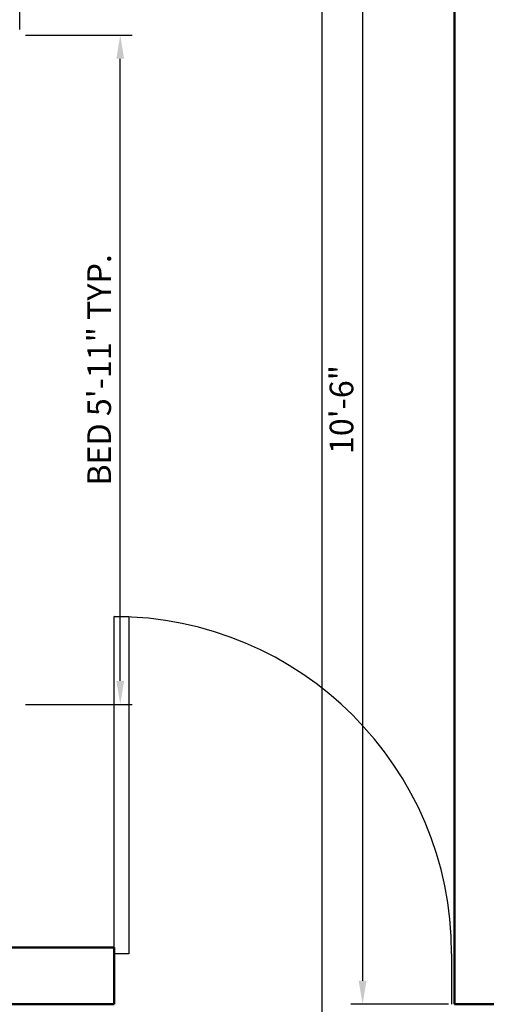
# Model space of a CAD drawing. Units: inches. Extents: x 2385 to 2740, y 1752 to 2305.
# Tile 9 of 15: x 2485 to 2535, y 2141 to 2245. Entities that reach past the tile are written whole.
import ezdxf

# ---------------------------------------------------------------- set-up
doc = ezdxf.new("R2010")
doc.units = ezdxf.units.IN
for name, color, linetype, lineweight in [('A-ANNO-DIMS', 2, 'Continuous', 18), ('A-DOOR', 4, 'Continuous', 25), ('A-WALL', 7, 'Continuous', 50)]:
    doc.layers.add(name, color=color, linetype=linetype, lineweight=lineweight)
doc.styles.get("Standard").update_dxf_attribs({"font": 'arial.ttf'})
doc.dimstyles.new('Copy of ISO-25', dxfattribs={"dimtxt": 2.5, "dimasz": 2.5, "dimexe": 1.25, "dimexo": 0.625, "dimtad": 1, "dimdec": 1, "dimlunit": 4, "dimtxsty": 'Standard', "dimcen": 2.5, "dimadec": 0, "dimazin": 0, "dimtfac": 1, "dimtdec": 1, "dimtmove": 0, "dimatfit": 3, "dimfxl": 1, "dimarcsym": 0})

# ---------------------------------------------------------------- blocks, each defined once
blk = doc.blocks.new('*D7')
at = {"layer": 'A-ANNO-DIMS', "color": 0, "lineweight": -2, "transparency": 16777216}
for p, q in [((2530.62, 2266.97), (2520.29, 2266.97)), ((2521.54, 2264.47), (2521.54, 2143.47)), ((2530.62, 2140.97), (2520.29, 2140.97))]:
    blk.add_line(p, q, dxfattribs=at)
at = {"layer": 'A-ANNO-DIMS', "color": 0, "transparency": 16777216}
for points in [[(2521.12, 2264.47), (2521.95, 2264.47), (2521.54, 2266.97)], [(2521.12, 2143.47), (2521.95, 2143.47), (2521.54, 2140.97)]]:
    blk.add_solid(points, dxfattribs=at)
at = {"layer": 'Defpoints', "color": 0, "transparency": 16777216}
for p in [(2531.25, 2266.97), (2521.54, 2140.97), (2531.25, 2140.97)]:
    blk.add_point(p, dxfattribs=at)
at = {"layer": 'A-ANNO-DIMS', "color": 0, "transparency": 16777216, "insert": (2519.63, 2203.97), "char_height": 2.5, "attachment_point": 5, "rotation": 90}
blk.add_mtext('10\'-6"', dxfattribs=at)
blk = doc.blocks.new('*U4')
for p, q in [((0, 0), (0, -6)), ((40, 0), (40, -6))]:
    blk.add_line(p, q)
blk.add_lwpolyline([(0, 0), (0, 40), (1.75, 40), (1.75, 0)], close=True)
blk.add_arc((0, 0), 40, 0, 90)
blk = doc.blocks.new('*D26')
at = {"layer": 'A-ANNO-DIMS', "color": 0, "lineweight": -2, "transparency": 16777216}
for p, q in [((2485.89, 2243.62), (2497.15, 2243.62)), ((2495.9, 2175.23), (2495.9, 2241.12)), ((2485.89, 2172.73), (2497.15, 2172.73))]:
    blk.add_line(p, q, dxfattribs=at)
at = {"layer": 'A-ANNO-DIMS', "color": 0, "transparency": 16777216}
for points in [[(2495.48, 2241.12), (2496.31, 2241.12), (2495.9, 2243.62)], [(2495.48, 2175.23), (2496.31, 2175.23), (2495.9, 2172.73)]]:
    blk.add_solid(points, dxfattribs=at)
at = {"layer": 'Defpoints', "color": 0, "transparency": 16777216}
for p in [(2485.26, 2243.62), (2495.9, 2243.62), (2485.26, 2172.73)]:
    blk.add_point(p, dxfattribs=at)
at = {"layer": 'A-ANNO-DIMS', "color": 0, "transparency": 16777216, "insert": (2493.99, 2208.17), "char_height": 2.5, "attachment_point": 5, "rotation": 90}
blk.add_mtext('BED 5\'-11" TYP.', dxfattribs=at)
blk = doc.blocks.new('*D27')
at = {"layer": 'A-ANNO-DIMS', "color": 0, "lineweight": -2, "transparency": 16777216}
for p, q in [((2429.86, 2244.24), (2429.86, 2255.5)), ((2485.26, 2244.24), (2485.26, 2255.5)), ((2482.76, 2254.25), (2432.36, 2254.25))]:
    blk.add_line(p, q, dxfattribs=at)
at = {"layer": 'A-ANNO-DIMS', "color": 0, "transparency": 16777216}
for points in [[(2432.36, 2254.67), (2432.36, 2253.84), (2429.86, 2254.25)], [(2482.76, 2254.67), (2482.76, 2253.84), (2485.26, 2254.25)]]:
    blk.add_solid(points, dxfattribs=at)
at = {"layer": 'Defpoints', "color": 0, "transparency": 16777216}
for p in [(2429.86, 2254.25), (2429.86, 2243.62), (2485.26, 2243.62)]:
    blk.add_point(p, dxfattribs=at)
at = {"layer": 'A-ANNO-DIMS', "color": 0, "transparency": 16777216, "insert": (2457.56, 2256.17), "char_height": 2.5, "attachment_point": 5}
blk.add_mtext('4\'-7 1/2" TYP.', dxfattribs=at)
blk = doc.blocks.new('*D48')
at = {"layer": 'A-ANNO-DIMS', "color": 0, "lineweight": -2, "transparency": 16777216}
for p, q in [((2517.25, 1916.59), (2517.25, 2302.84)), ((2553.25, 1916.59), (2553.25, 2302.84)), ((2519.75, 2301.59), (2550.75, 2301.59))]:
    blk.add_line(p, q, dxfattribs=at)
at = {"layer": 'A-ANNO-DIMS', "color": 0, "transparency": 16777216}
for points in [[(2519.75, 2302), (2519.75, 2301.17), (2517.25, 2301.59)], [(2550.75, 2302), (2550.75, 2301.17), (2553.25, 2301.59)]]:
    blk.add_solid(points, dxfattribs=at)
at = {"layer": 'Defpoints', "color": 0, "transparency": 16777216}
for p in [(2553.25, 2301.59), (2517.25, 1915.97), (2553.25, 1915.97)]:
    blk.add_point(p, dxfattribs=at)
at = {"layer": 'A-ANNO-DIMS', "color": 0, "transparency": 16777216, "insert": (2535.25, 2303.49), "char_height": 2.5, "attachment_point": 5}
blk.add_mtext('3\'-0"', dxfattribs=at)

msp = doc.modelspace()

# ---------------------------------------------------------------- linework, layer by layer
at = {"layer": 'A-WALL'}
for p, q in [((2531.25, 2146.97), (2531.25, 2266.97)), ((2423.25, 2146.97), (2495.25, 2146.97)), ((2495.25, 2140.97), (2495.25, 2146.97)), ((2531.25, 2146.97), (2531.25, 2140.97)), ((2495.25, 2140.97), (2423.25, 2140.97)), ((2583.25, 2140.97), (2531.25, 2140.97))]:
    msp.add_line(p, q, dxfattribs=at)

# ---------------------------------------------------------------- block references
at = {"layer": 'A-DOOR', "xscale": 0.8927336239432367, "yscale": 0.8927336239432367, "zscale": 0.8927336239432367}
msp.add_blockref('*U4', (2495.25, 2146.33), dxfattribs=at)

# ---------------------------------------------------------------- dimensions: what is measured, and where the dimension line sits
at = {"layer": 'A-ANNO-DIMS'}
dim = msp.add_linear_dim(base=(2553.25, 2301.59), p1=(2517.25, 1915.97), p2=(2553.25, 1915.97), dimstyle='Copy of ISO-25', override={"dimdec": 1, "dimlfac": 1, "dimrnd": 0, "dimzin": 1, "dimdsep": 46, "dimlunit": 4, "dimfrac": 2}, dxfattribs=at)
dim.commit()
dim.dimension.update_dxf_attribs({"geometry": '*D48', "text_midpoint": (2535.25, 2303.49)})
dim = msp.add_linear_dim(base=(2521.54, 2140.97), p1=(2531.25, 2266.97), p2=(2531.25, 2140.97), angle=90, dimstyle='Copy of ISO-25', override={"dimclrd": 0, "dimclre": 0, "dimclrt": 0}, dxfattribs=at)
dim.commit()
dim.dimension.update_dxf_attribs({"geometry": '*D7', "text_midpoint": (2519.63, 2203.97)})
for base, p1, p2, angle, text, picture, middle in [((2429.86, 2254.25), (2485.26, 2243.62), (2429.86, 2243.62), 180, '<> TYP.', '*D27', (2457.56, 2256.17)), ((2495.9, 2243.62), (2485.26, 2172.73), (2485.26, 2243.62), 90, 'BED <> TYP.', '*D26', (2493.99, 2208.17))]:
    dim = msp.add_linear_dim(base=base, p1=p1, p2=p2, angle=angle, text=text, dimstyle='Copy of ISO-25', override={"dimdec": 1, "dimlfac": 1, "dimrnd": 0, "dimzin": 1, "dimdsep": 46, "dimlunit": 4, "dimfrac": 2}, dxfattribs=at)
    dim.commit()
    dim.dimension.update_dxf_attribs({"geometry": picture, "text_midpoint": middle})

doc.saveas('drawing.dxf')
